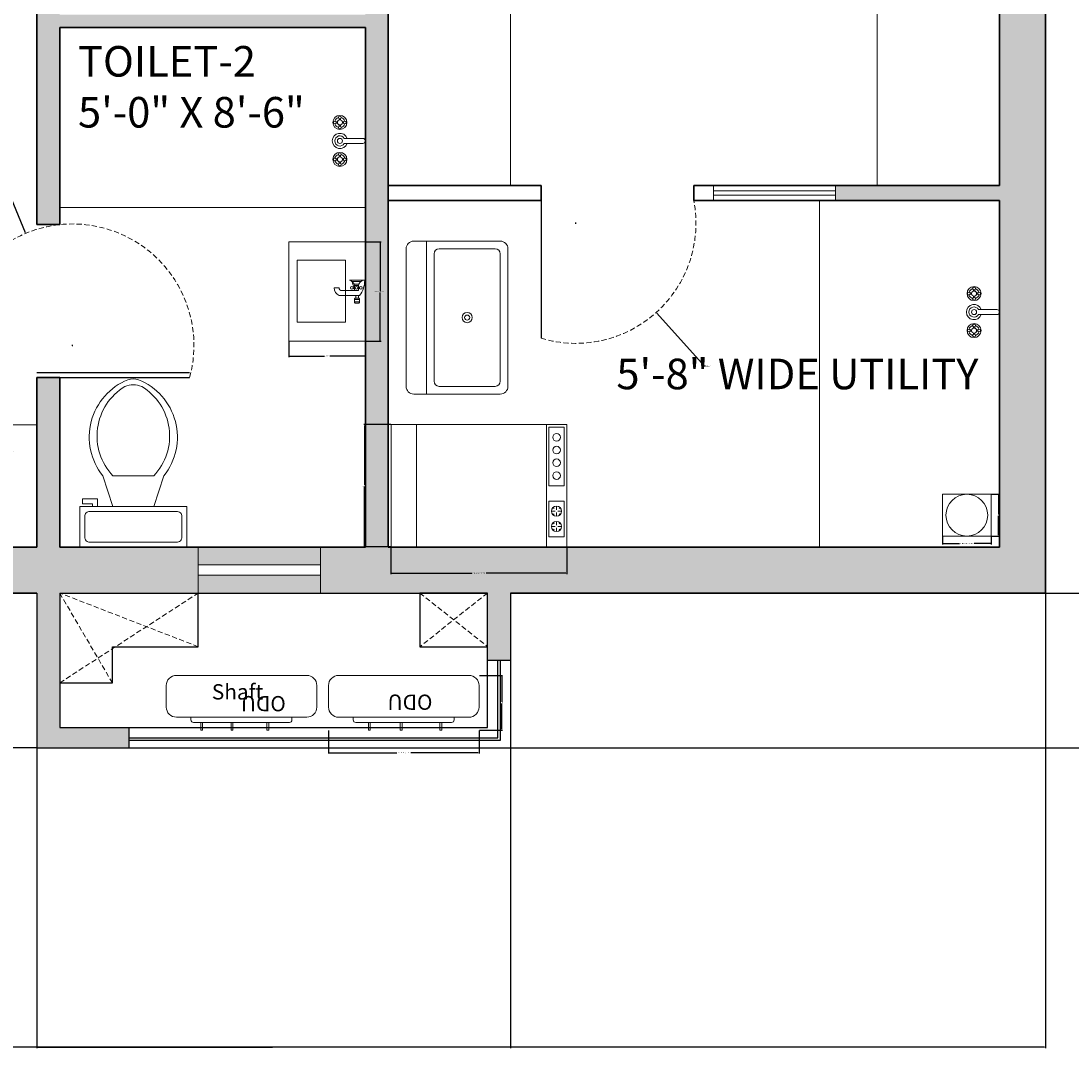
# Model space of a CAD drawing. Units: inches. Extents: x 1693 to 2974, y 2201 to 2965.
# Tile 9 of 24: x 2093 to 2299, y 2201 to 2402. Entities that reach past the tile are written whole.
import ezdxf

# ---------------------------------------------------------------- set-up
doc = ezdxf.new("R2010")
doc.units = ezdxf.units.IN
doc.header["$LTSCALE"] = 2
doc.header["$MEASUREMENT"] = 0
doc.linetypes.add('HIDDEN', pattern=[0.375, 0.25, -0.125])
for name, color, linetype, lineweight in [('A-ANNO-DIMS', 2, 'Continuous', 18), ('A-ANNO-TEXT', 7, 'Continuous', 13), ('A-AREA-IDEN', 7, 'Continuous', 18), ('A-DOOR', 3, 'Continuous', 25), ('A-DOOR-SWNG', 3, 'HIDDEN', 13), ('A-EQPM', 8, 'Continuous', 18), ('A-FLOR-CASE', 32, 'Continuous', 18), ('A-FLOR-FIXT', 9, 'Continuous', 18), ('A-FLOR-SHFT', 7, 'Continuous', 25), ('A-FLOR-SHFT-HIDN', 8, 'HIDDEN', 13), ('A-GLAZ', 4, 'Continuous', 18), ('A-WALL', 7, 'Continuous', 35), ('M-HVAC-EQPM', 151, 'Continuous', 18)]:
    doc.layers.add(name, color=color, linetype=linetype, lineweight=lineweight)
doc.layers.add('A-GLAZ-PATT', color=141, linetype='Continuous', lineweight=13, true_color=0xadddf7)
doc.layers.add('A-WALL-PATT', color=251, linetype='Continuous', lineweight=13, true_color=0x636466)
doc.styles.get("Standard").update_dxf_attribs({"font": 'arial.ttf'})
doc.dimstyles.get("Standard").update_dxf_attribs({"dimtxt": 0.18, "dimasz": 0.18, "dimexe": 0.18, "dimexo": 0.0625, "dimgap": 0.09, "dimtad": 0, "dimtih": 1, "dimtoh": 1, "dimdec": 1, "dimzin": 0, "dimdsep": 46, "dimlunit": 3, "dimtxsty": 'Standard', "dimcen": 0.09, "dimadec": 0, "dimazin": 0, "dimtfac": 1, "dimtdec": 1, "dimtofl": 0, "dimtmove": 0, "dimatfit": 3, "dimfxl": 1, "dimtolj": 1, "dimtzin": 0, "dimarcsym": 0})

# ---------------------------------------------------------------- blocks, each defined once
blk = doc.blocks.new('Faucet - Bathroom top')
for p, q in [((-4.107, 0.125), (-4.375, 0.125)), ((-3.75, 0.4788), (-3.75, 0.75)), ((-3.5, 0.482), (-3.5, 0.75)), ((-3.1461, 0.125), (-2.875, 0.125)), ((3.143, 0.125), (2.875, 0.125)), ((3.5, 0.4788), (3.5, 0.75)), ((3.75, 0.482), (3.75, 0.75)), ((4.1039, 0.125), (4.375, 0.125)), ((-4.1039, -0.125), (-4.375, -0.125)), ((-3.75, -0.4821), (-3.75, -0.75)), ((-3.5, -0.4789), (-3.5, -0.75)), ((-3.143, -0.125), (-2.875, -0.125)), ((-0.5, -0.8639), (-0.5, -4.5)), ((0.5, -4.5), (0.5, -0.8631)), ((3.1461, -0.125), (2.875, -0.125)), ((3.5, -0.4821), (3.5, -0.75)), ((3.75, -0.4789), (3.75, -0.75)), ((4.107, -0.125), (4.375, -0.125))]:
    blk.add_line(p, q)
for centre, radius in [((-3.625, 0), 1.375), ((-4.625, 0), 0.2795), ((-3.625, 0), 0.5), ((-3.625, 1), 0.2795), ((-2.625, 0), 0.2795), ((0, 0), 0.5), ((3.625, 0), 1.375), ((2.625, 0), 0.2795), ((3.625, 0), 0.5), ((3.625, 1), 0.2795), ((4.625, 0), 0.2795), ((-3.625, -1), 0.2795), ((3.625, -1), 0.2795)]:
    blk.add_circle(centre, radius)
for centre, radius, start, end in [((-3.625, 0), 1, 105.2407, 164.2093), ((-3.625, 0), 1, 16.44125, 74.07887), ((0, 0), 1.5, 289.6514, 250.3603), ((0, 0), 1, 300.3431, 239.7554), ((3.625, 0), 1, 106.12, 164.0884), ((3.625, 0), 1, 16.23422, 73.90469), ((-3.625, 0), 1, 196.2342, 253.9047), ((-3.625, 0), 1, 286.12, 344.0884), ((3.625, 0), 1, 196.4413, 254.0789), ((3.625, 0), 1, 285.2407, 344.2093), ((0, -4.5), 0.5, 180, 0)]:
    blk.add_arc(centre, radius, start, end)
blk = doc.blocks.new('Faucet - Bathroom side')
for p, q in [((-0.625, 4.25), (0.375, 4.25)), ((0.375, 3.75), (-0.625, 3.75)), ((-0.625, 3), (3.375, 3)), ((-0.375, 3), (-0.375, 3.5)), ((0.125, 3.5), (0.125, 3)), ((-1.625, 0), (-1.375, 0)), ((-1.375, 0), (1.375, 0)), ((-0.88366, 0.25), (0.88424, 0.25)), ((-0.375, 1.625), (-0.625, 1.625)), ((-0.375, 1.375), (-0.625, 1.375)), ((0.48078, 0.75), (-0.47286, 0.75)), ((2.875, 2), (0.375, 2)), ((0.375, 1.625), (0.625, 1.625)), ((0.375, 1.375), (0.625, 1.375)), ((4.375, 1.5), (3.375, 1.5))]:
    blk.add_line(p, q)
for points in [[(-0.625, 3.75), (-0.625, 4.25)], [(-0.375, 4.5), (0.125, 4.5)], [(0.375, 4.25), (0.375, 3.75)], [(0.125, 3.5), (-0.375, 3.5)]]:
    blk.add_lwpolyline(points)
blk.add_lwpolyline([(-0.375, 1), (-0.375, 2), (0.375, 2), (0.375, 1)], close=True)
for centre in [(-0.875, 1.5), (0, 1.5), (0.875, 1.5)]:
    blk.add_circle(centre, 0.27951)
for centre, radius, start, end in [((-0.38253, 4.2575), 0.24259, 88.22243, 181.7776), ((0.13252, 4.2575), 0.24259, 358.2224, 91.77757), ((3.45929, -0.0281), 5.08436, 143.4467, 179.6834), ((-0.38253, 3.7424), 0.24259, 178.2224, 271.7776), ((0.13252, 3.7424), 0.24259, 268.2224, 1.777565), ((2.70708, 1.4714), 1.66816, 0.9827695, 66.39737), ((-1.75, 1.375), 1.42522, 285.2551, 344.7449), ((1.75, 1.375), 1.42522, 195.2551, 254.7449), ((-2.49562, -0.286), 3.38273, 9.709485, 29.48735), ((2.96867, 1.5936), 0.41699, 347.0192, 102.9808)]:
    blk.add_arc(centre, radius, start, end)
blk = doc.blocks.new('Toilet - top')
for p, q in [((9.5, -6), (9.5, -2)), ((-8, -8.5), (-8, -8)), ((-7, -8), (-7, -9.5)), ((-4, -8), (-6, -14)), ((4, -8), (6, -14)), ((-10, -8.5), (-8, -8.5)), ((-10, -9.5), (-10, -8.5)), ((-7, -9.5), (-10, -9.5)), ((4, -14), (-4, -14))]:
    blk.add_line(p, q)
blk.add_lwpolyline([(10.5, -8), (10.5, 0), (-10.5, 0), (-10.5, -8)], close=True)
for points in [[(-9.5, -2), (-9.5, -6)], [(8.5, -1), (-8.5, -1)], [(-8.5, -7), (8.5, -7)]]:
    blk.add_lwpolyline(points)
for centre, radius, start, end in [((-8.62, -1.88), 0.884, 81.8699, 188.1301), ((8.62, -1.88), 0.884, 351.8699, 98.1301), ((-8.62, -6.12), 0.884, 171.8699, 278.1301), ((8.62, -6.12), 0.884, 261.8699, 8.1301), ((3.52, -21.58), 12.17, 141.4691, 247.9714), ((4.2, -21.82), 11.33, 136.3677, 238.9468), ((-3.52, -21.58), 12.17, 292.0284, 38.5307), ((-4.2, -21.82), 11.33, 301.053, 43.6321), ((0, -27.88), 4, 245.7318, 294.2682), ((0, -29), 4, 254.8605, 285.1395)]:
    blk.add_arc(centre, radius, start, end)
blk = doc.blocks.new('Dishwasher')
for p, q in [((16.3156, 33.1843), (16.5, 33)), ((17, 32.75), (17, 33.5)), ((17.5, 33), (17.6938, 33.1938)), ((19.3156, 33.1843), (19.5, 33)), ((20, 32.75), (20, 33.5)), ((20.5, 33), (20.6938, 33.1938)), ((16, 32.5), (16.75, 32.5)), ((16.5, 32), (16.2942, 31.7942)), ((17, 32.25), (17, 31.5)), ((18, 32.5), (17.25, 32.5)), ((17.7061, 31.7939), (17.5, 32)), ((19, 32.5), (19.75, 32.5)), ((19.5, 32), (19.2942, 31.7942)), ((20, 32.25), (20, 31.5)), ((21, 32.5), (20.25, 32.5)), ((20.7061, 31.7939), (20.5, 32)), ((24, 30.5), (0, 30.5)), ((0, 5), (24, 5))]:
    blk.add_line(p, q)
for points in [[(0, 0), (0, 34.5), (24, 34.5), (24, 0)], [(0.5, 31), (0.5, 34), (12, 34), (12, 31)], [(15, 31), (15, 34), (22, 34), (22, 31)]]:
    blk.add_lwpolyline(points, close=True)
for centre, radius in [((2.5, 32.5), 0.75), ((5, 32.5), 0.75), ((7.5, 32.5), 0.75), ((10, 32.5), 0.75), ((17, 32.5), 1), ((20, 32.5), 1)]:
    blk.add_circle(centre, radius)
blk = doc.blocks.new('Sink-single - 30 in top')
blk.add_line((-15, -3.999996), (15, -3.999996))
for points in [[(-13.5, 0), (13.5, 0)], [(-15, -18.499996), (-15, -1.5)], [(15, -1.5), (15, -18.499996)], [(-12.5, -5.499996), (12.5, -5.499996)], [(-13.5, -17.499996), (-13.5, -6.499996)], [(13.5, -6.499996), (13.5, -17.499996)], [(12.5, -18.499996), (-12.5, -18.499996)], [(13.5, -19.999996), (-13.5, -19.999996)]]:
    blk.add_lwpolyline(points)
for radius in [1, 0.5]:
    blk.add_circle((0, -11.999996), radius)
for centre, radius, start, end in [((-13.5, -1.5), 1.5, 90, 180), ((13.5, -1.5), 1.5, 0, 90), ((-12.5, -6.499996), 1, 90, 180), ((12.5, -6.499996), 1, 0, 90), ((-13.5, -18.499996), 1.5, 180, 270), ((-12.5, -17.499996), 1, 180, 270), ((12.5, -17.499996), 1, 270, 0), ((13.5, -18.499996), 1.5, 270, 0)]:
    blk.add_arc(centre, radius, start, end)
blk = doc.blocks.new('BASIN-WALL-MOUNT')
at = {"ltscale": 2}
for points in [[(15.01, 19.49), (0, 19.49), (0, 0), (15.01, 0)], [(11.1, 15.94), (1.63, 15.94), (1.63, 3.76), (11.1, 3.76)]]:
    blk.add_lwpolyline(points, close=True, dxfattribs=at)
blk = doc.blocks.new('DRAIN-UTILITY')
at = {"ltscale": 2}
blk.add_lwpolyline([(0, 8.21), (9.59, 8.21), (9.59, 0), (0, 0)], close=True, dxfattribs=at)
blk.add_circle((4.8, 4.1), 4.1, dxfattribs=at)
blk = doc.blocks.new('CONDENSER-WITH-BRACKETS')
at = {"ltscale": 2}
for points in [[(2, 10.74), (27.57, 10.74, -0.414214), (29.57, 8.74), (29.57, 4.53, -0.414214), (27.57, 2.53), (2, 2.53, -0.414214), (0, 4.53), (0, 8.74, -0.414214)], [(4.85, 2.53), (24.67, 2.53), (24.67, 2, -0.414214), (24.17, 1.5), (5.35, 1.5, -0.414214), (4.85, 2)]]:
    blk.add_lwpolyline(points, format="xyb", close=True, dxfattribs=at)
for points in [[(7.84, 1.5), (8.19, 1.5), (8.19, 0), (7.84, 0)], [(14.1, 1.5), (14.45, 1.5), (14.45, 0), (14.1, 0)], [(21.89, 1.5), (22.24, 1.5), (22.24, 0), (21.89, 0)]]:
    blk.add_lwpolyline(points, close=True, dxfattribs=at)
blk = doc.blocks.new('*D43')
at = {"layer": 'A-ANNO-DIMS', "color": 0, "lineweight": -2, "ltscale": 2, "transparency": 16777216}
for p, q in [((2160.8, 2358.73), (2163.84, 2358.73)), ((2163.66, 2358.55), (2163.66, 2349.17)), ((2163.66, 2339.42), (2163.66, 2348.8)), ((2160.8, 2339.24), (2163.84, 2339.24))]:
    blk.add_line(p, q, dxfattribs=at)
at = {"layer": 'A-ANNO-DIMS', "color": 0, "ltscale": 2, "transparency": 16777216}
for points in [[(2163.63, 2358.55), (2163.69, 2358.55), (2163.66, 2358.73)], [(2163.63, 2339.42), (2163.69, 2339.42), (2163.66, 2339.24)]]:
    blk.add_solid(points, dxfattribs=at)
at = {"layer": 'Defpoints', "color": 0, "ltscale": 2, "transparency": 16777216}
for p in [(2160.74, 2358.73), (2163.66, 2358.73), (2160.74, 2339.24)]:
    blk.add_point(p, dxfattribs=at)
at = {"layer": 'A-ANNO-DIMS', "color": 0, "ltscale": 2, "transparency": 16777216, "insert": (2163.66, 2348.98), "char_height": 0.18, "attachment_point": 5}
blk.add_mtext('\\A1;WALL BASIN 19 TYP.', dxfattribs=at)
blk = doc.blocks.new('*D44')
at = {"layer": 'A-ANNO-DIMS', "color": 0, "lineweight": -2, "ltscale": 2, "transparency": 16777216}
for p, q in [((2145.72, 2339.18), (2145.72, 2336.13)), ((2160.74, 2339.18), (2160.74, 2336.13)), ((2145.9, 2336.31), (2152.71, 2336.31)), ((2160.56, 2336.31), (2153.75, 2336.31))]:
    blk.add_line(p, q, dxfattribs=at)
at = {"layer": 'A-ANNO-DIMS', "color": 0, "ltscale": 2, "transparency": 16777216}
for points in [[(2145.9, 2336.34), (2145.9, 2336.28), (2145.72, 2336.31)], [(2160.56, 2336.34), (2160.56, 2336.28), (2160.74, 2336.31)]]:
    blk.add_solid(points, dxfattribs=at)
at = {"layer": 'Defpoints', "color": 0, "ltscale": 2, "transparency": 16777216}
for p in [(2145.72, 2339.24), (2160.74, 2339.24), (2160.74, 2336.31)]:
    blk.add_point(p, dxfattribs=at)
at = {"layer": 'A-ANNO-DIMS', "color": 0, "ltscale": 2, "transparency": 16777216, "insert": (2153.23, 2336.31), "char_height": 0.18, "attachment_point": 5}
blk.add_mtext('\\A1;15 TYP.', dxfattribs=at)
blk = doc.blocks.new('*D57')
at = {"layer": 'A-ANNO-DIMS', "color": 0, "lineweight": -2, "ltscale": 2, "transparency": 16777216}
for p, q in [((2165.77, 2298.84), (2165.77, 2293.55)), ((2200.27, 2298.84), (2200.27, 2293.55)), ((2165.95, 2293.73), (2181.61, 2293.73)), ((2200.09, 2293.73), (2184.44, 2293.73))]:
    blk.add_line(p, q, dxfattribs=at)
at = {"layer": 'A-ANNO-DIMS', "color": 0, "ltscale": 2, "transparency": 16777216}
for points in [[(2165.95, 2293.76), (2165.95, 2293.7), (2165.77, 2293.73)], [(2200.09, 2293.76), (2200.09, 2293.7), (2200.27, 2293.73)]]:
    blk.add_solid(points, dxfattribs=at)
at = {"layer": 'Defpoints', "color": 0, "ltscale": 2, "transparency": 16777216}
for p in [(2165.77, 2298.9), (2200.27, 2298.9), (2200.27, 2293.73)]:
    blk.add_point(p, dxfattribs=at)
at = {"layer": 'A-ANNO-DIMS', "color": 0, "ltscale": 2, "transparency": 16777216, "insert": (2183.02, 2293.73), "char_height": 0.18, "attachment_point": 5}
blk.add_mtext('\\A1;DISHWASHER 35 TYP.', dxfattribs=at)
blk = doc.blocks.new('*D58')
at = {"layer": 'A-ANNO-DIMS', "color": 0, "lineweight": -2, "ltscale": 2, "transparency": 16777216}
for p, q in [((2165.71, 2322.9), (2160.42, 2322.9)), ((2160.6, 2322.72), (2160.6, 2311.08)), ((2160.6, 2299.08), (2160.6, 2310.72)), ((2165.71, 2298.9), (2160.42, 2298.9))]:
    blk.add_line(p, q, dxfattribs=at)
at = {"layer": 'A-ANNO-DIMS', "color": 0, "ltscale": 2, "transparency": 16777216}
for points in [[(2160.57, 2322.72), (2160.63, 2322.72), (2160.6, 2322.9)], [(2160.57, 2299.08), (2160.63, 2299.08), (2160.6, 2298.9)]]:
    blk.add_solid(points, dxfattribs=at)
at = {"layer": 'Defpoints', "color": 0, "ltscale": 2, "transparency": 16777216}
for p in [(2165.77, 2322.9), (2160.6, 2298.9), (2165.77, 2298.9)]:
    blk.add_point(p, dxfattribs=at)
at = {"layer": 'A-ANNO-DIMS', "color": 0, "ltscale": 2, "transparency": 16777216, "insert": (2160.6, 2310.9), "char_height": 0.18, "attachment_point": 5}
blk.add_mtext('\\A1;24 TYP.', dxfattribs=at)
blk = doc.blocks.new('*D77')
at = {"layer": 'A-ANNO-DIMS', "color": 0, "lineweight": -2, "ltscale": 2, "transparency": 16777216}
for p, q in [((2274.03, 2300.96), (2274.03, 2299.4)), ((2283.62, 2300.96), (2283.62, 2299.4)), ((2274.21, 2299.58), (2277.37, 2299.58)), ((2283.44, 2299.58), (2280.28, 2299.58))]:
    blk.add_line(p, q, dxfattribs=at)
at = {"layer": 'A-ANNO-DIMS', "color": 0, "ltscale": 2, "transparency": 16777216}
for points in [[(2274.21, 2299.61), (2274.21, 2299.55), (2274.03, 2299.58)], [(2283.44, 2299.61), (2283.44, 2299.55), (2283.62, 2299.58)]]:
    blk.add_solid(points, dxfattribs=at)
at = {"layer": 'Defpoints', "color": 0, "ltscale": 2, "transparency": 16777216}
for p in [(2274.03, 2301.02), (2283.62, 2301.02), (2283.62, 2299.58)]:
    blk.add_point(p, dxfattribs=at)
at = {"layer": 'A-ANNO-DIMS', "color": 0, "ltscale": 2, "transparency": 16777216, "insert": (2278.82, 2299.58), "char_height": 0.18, "attachment_point": 5}
blk.add_mtext('\\A1;UTILITY DRAIN 10 TYP.', dxfattribs=at)
blk = doc.blocks.new('*D78')
at = {"layer": 'A-ANNO-DIMS', "color": 0, "lineweight": -2, "ltscale": 2, "transparency": 16777216}
for p, q in [((2283.68, 2309.23), (2285.24, 2309.23)), ((2285.06, 2309.05), (2285.06, 2305.31)), ((2285.06, 2301.2), (2285.06, 2304.94)), ((2283.68, 2301.02), (2285.24, 2301.02))]:
    blk.add_line(p, q, dxfattribs=at)
at = {"layer": 'A-ANNO-DIMS', "color": 0, "ltscale": 2, "transparency": 16777216}
for points in [[(2285.03, 2309.05), (2285.09, 2309.05), (2285.06, 2309.23)], [(2285.03, 2301.2), (2285.09, 2301.2), (2285.06, 2301.02)]]:
    blk.add_solid(points, dxfattribs=at)
at = {"layer": 'Defpoints', "color": 0, "ltscale": 2, "transparency": 16777216}
for p in [(2283.62, 2309.23), (2285.06, 2309.23), (2283.62, 2301.02)]:
    blk.add_point(p, dxfattribs=at)
at = {"layer": 'A-ANNO-DIMS', "color": 0, "ltscale": 2, "transparency": 16777216, "insert": (2285.06, 2305.12), "char_height": 0.18, "attachment_point": 5}
blk.add_mtext('\\A1;8 TYP.', dxfattribs=at)
blk = doc.blocks.new('*D79')
at = {"layer": 'A-ANNO-DIMS', "color": 0, "lineweight": -2, "ltscale": 2, "transparency": 16777216}
for p, q in [((2153.5, 2262.88), (2153.5, 2258.33)), ((2183.07, 2262.88), (2183.07, 2258.33)), ((2153.68, 2258.51), (2166.92, 2258.51)), ((2182.89, 2258.51), (2169.65, 2258.51))]:
    blk.add_line(p, q, dxfattribs=at)
at = {"layer": 'A-ANNO-DIMS', "color": 0, "ltscale": 2, "transparency": 16777216}
for points in [[(2153.68, 2258.54), (2153.68, 2258.48), (2153.5, 2258.51)], [(2182.89, 2258.54), (2182.89, 2258.48), (2183.07, 2258.51)]]:
    blk.add_solid(points, dxfattribs=at)
at = {"layer": 'Defpoints', "color": 0, "ltscale": 2, "transparency": 16777216}
for p in [(2153.5, 2262.95), (2183.07, 2262.95), (2183.07, 2258.51)]:
    blk.add_point(p, dxfattribs=at)
at = {"layer": 'A-ANNO-DIMS', "color": 0, "ltscale": 2, "transparency": 16777216, "insert": (2168.28, 2258.51), "char_height": 0.18, "attachment_point": 5}
blk.add_mtext('\\A1;CONDENSER 30 TYP.', dxfattribs=at)
blk = doc.blocks.new('*D80')
at = {"layer": 'A-ANNO-DIMS', "color": 0, "lineweight": -2, "ltscale": 2, "transparency": 16777216}
for p, q in [((2183.13, 2273.69), (2187.68, 2273.69)), ((2187.5, 2273.51), (2187.5, 2268.5)), ((2187.5, 2263.13), (2187.5, 2268.14)), ((2183.13, 2262.95), (2187.68, 2262.95))]:
    blk.add_line(p, q, dxfattribs=at)
at = {"layer": 'A-ANNO-DIMS', "color": 0, "ltscale": 2, "transparency": 16777216}
for points in [[(2187.47, 2273.51), (2187.53, 2273.51), (2187.5, 2273.69)], [(2187.47, 2263.13), (2187.53, 2263.13), (2187.5, 2262.95)]]:
    blk.add_solid(points, dxfattribs=at)
at = {"layer": 'Defpoints', "color": 0, "ltscale": 2, "transparency": 16777216}
for p in [(2183.07, 2273.69), (2187.5, 2273.69), (2183.07, 2262.95)]:
    blk.add_point(p, dxfattribs=at)
at = {"layer": 'A-ANNO-DIMS', "color": 0, "ltscale": 2, "transparency": 16777216, "insert": (2187.5, 2268.32), "char_height": 0.18, "attachment_point": 5}
blk.add_mtext('\\A1;11 TYP.', dxfattribs=at)
blk = doc.blocks.new('*D82')
at = {"layer": 'A-ANNO-DIMS', "color": 0, "lineweight": -2, "ltscale": 2, "transparency": 16777216}
for p, q in [((2615.67, 2906.08), (1693.46, 2906.08)), ((1693.64, 2905.9), (1693.64, 2582.94)), ((1693.64, 2259.62), (1693.64, 2582.58)), ((2096.17, 2259.44), (1693.46, 2259.44))]:
    blk.add_line(p, q, dxfattribs=at)
at = {"layer": 'A-ANNO-DIMS', "color": 0, "ltscale": 2, "transparency": 16777216}
for points in [[(1693.61, 2905.9), (1693.67, 2905.9), (1693.64, 2906.08)], [(1693.61, 2259.62), (1693.67, 2259.62), (1693.64, 2259.44)]]:
    blk.add_solid(points, dxfattribs=at)
at = {"layer": 'Defpoints', "color": 0, "ltscale": 2, "transparency": 16777216}
for p in [(1693.64, 2906.08), (2615.74, 2906.08), (2096.24, 2259.44)]:
    blk.add_point(p, dxfattribs=at)
at = {"layer": 'A-ANNO-DIMS', "color": 0, "ltscale": 2, "transparency": 16777216, "insert": (1693.64, 2582.76), "char_height": 0.18, "attachment_point": 5}
blk.add_mtext('\\A1;646.6', dxfattribs=at)
blk = doc.blocks.new('*D83')
at = {"layer": 'A-ANNO-DIMS', "color": 0, "lineweight": -2, "ltscale": 2, "transparency": 16777216}
for p, q in [((1782.74, 2289.78), (1782.74, 2200.56)), ((2294.24, 2289.78), (2294.24, 2200.56)), ((1782.92, 2200.74), (2038.09, 2200.74)), ((2294.06, 2200.74), (2038.88, 2200.74))]:
    blk.add_line(p, q, dxfattribs=at)
at = {"layer": 'A-ANNO-DIMS', "color": 0, "ltscale": 2, "transparency": 16777216}
for points in [[(1782.92, 2200.77), (1782.92, 2200.71), (1782.74, 2200.74)], [(2294.06, 2200.77), (2294.06, 2200.71), (2294.24, 2200.74)]]:
    blk.add_solid(points, dxfattribs=at)
at = {"layer": 'Defpoints', "color": 0, "ltscale": 2, "transparency": 16777216}
for p in [(1782.74, 2289.84), (2294.24, 2289.84), (2294.24, 2200.74)]:
    blk.add_point(p, dxfattribs=at)
at = {"layer": 'A-ANNO-DIMS', "color": 0, "ltscale": 2, "transparency": 16777216, "insert": (2038.49, 2200.74), "char_height": 0.18, "attachment_point": 5}
blk.add_mtext('\\A1;511.5', dxfattribs=at)
blk = doc.blocks.new('*D89')
at = {"layer": 'A-ANNO-DIMS', "color": 0, "lineweight": -2, "ltscale": 2, "transparency": 16777216}
for p, q in [((2479.3, 2334.75), (2973.12, 2334.75)), ((2972.94, 2334.57), (2972.94, 2312.48)), ((2972.94, 2290.02), (2972.94, 2312.12)), ((2294.3, 2289.84), (2973.12, 2289.84))]:
    blk.add_line(p, q, dxfattribs=at)
at = {"layer": 'A-ANNO-DIMS', "color": 0, "ltscale": 2, "transparency": 16777216}
for points in [[(2972.91, 2334.57), (2972.97, 2334.57), (2972.94, 2334.75)], [(2972.91, 2290.02), (2972.97, 2290.02), (2972.94, 2289.84)]]:
    blk.add_solid(points, dxfattribs=at)
at = {"layer": 'Defpoints', "color": 0, "ltscale": 2, "transparency": 16777216}
for p in [(2479.24, 2334.75), (2972.94, 2334.75), (2294.24, 2289.84)]:
    blk.add_point(p, dxfattribs=at)
at = {"layer": 'A-ANNO-DIMS', "color": 0, "ltscale": 2, "transparency": 16777216, "insert": (2972.94, 2312.3), "char_height": 0.18, "attachment_point": 5}
blk.add_mtext('\\A1;44.91', dxfattribs=at)
blk = doc.blocks.new('*D94')
at = {"layer": 'A-ANNO-DIMS', "color": 0, "lineweight": -2, "ltscale": 2, "transparency": 16777216}
for p, q in [((2096.24, 2259.38), (2096.24, 2200.56)), ((2189.24, 2259.38), (2189.24, 2200.56)), ((2096.42, 2200.74), (2142.52, 2200.74)), ((2189.06, 2200.74), (2142.96, 2200.74))]:
    blk.add_line(p, q, dxfattribs=at)
at = {"layer": 'A-ANNO-DIMS', "color": 0, "ltscale": 2, "transparency": 16777216}
for points in [[(2096.42, 2200.77), (2096.42, 2200.71), (2096.24, 2200.74)], [(2189.06, 2200.77), (2189.06, 2200.71), (2189.24, 2200.74)]]:
    blk.add_solid(points, dxfattribs=at)
at = {"layer": 'Defpoints', "color": 0, "ltscale": 2, "transparency": 16777216}
for p in [(2096.24, 2259.44), (2189.24, 2259.44), (2189.24, 2200.74)]:
    blk.add_point(p, dxfattribs=at)
at = {"layer": 'A-ANNO-DIMS', "color": 0, "ltscale": 2, "transparency": 16777216, "insert": (2142.74, 2200.74), "char_height": 0.18, "attachment_point": 5}
blk.add_mtext('\\A1;93', dxfattribs=at)
blk = doc.blocks.new('*D95')
at = {"layer": 'A-ANNO-DIMS', "color": 0, "lineweight": -2, "ltscale": 2, "transparency": 16777216}
for p, q in [((2189.3, 2289.84), (2973.12, 2289.84)), ((2972.94, 2289.66), (2972.94, 2274.83)), ((2972.94, 2259.62), (2972.94, 2274.46)), ((2189.3, 2259.44), (2973.12, 2259.44))]:
    blk.add_line(p, q, dxfattribs=at)
at = {"layer": 'A-ANNO-DIMS', "color": 0, "ltscale": 2, "transparency": 16777216}
for points in [[(2972.91, 2289.66), (2972.97, 2289.66), (2972.94, 2289.84)], [(2972.91, 2259.62), (2972.97, 2259.62), (2972.94, 2259.44)]]:
    blk.add_solid(points, dxfattribs=at)
at = {"layer": 'Defpoints', "color": 0, "ltscale": 2, "transparency": 16777216}
for p in [(2189.24, 2289.84), (2972.94, 2289.84), (2189.24, 2259.44)]:
    blk.add_point(p, dxfattribs=at)
at = {"layer": 'A-ANNO-DIMS', "color": 0, "ltscale": 2, "transparency": 16777216, "insert": (2972.94, 2274.64), "char_height": 0.18, "attachment_point": 5}
blk.add_mtext('\\A1;30.4', dxfattribs=at)
blk = doc.blocks.new('*D126')
at = {"layer": 'A-ANNO-DIMS', "color": 0, "lineweight": -2, "ltscale": 2, "transparency": 16777216}
for p, q in [((2088.31, 2373.6), (2088.49, 2373.6)), ((2088.49, 2373.6), (2093.95, 2360.58)), ((2103.15, 2338.43), (2103.33, 2338.43)), ((2103.24, 2338.34), (2103.24, 2338.52))]:
    blk.add_line(p, q, dxfattribs=at)
at = {"layer": 'A-ANNO-DIMS', "color": 0, "ltscale": 2, "transparency": 16777216}
blk.add_solid([(2093.98, 2360.59), (2093.93, 2360.57), (2094.02, 2360.41)], dxfattribs=at)
at = {"layer": 'Defpoints', "color": 0, "ltscale": 2, "transparency": 16777216}
for p in [(2094.02, 2360.41), (2103.24, 2338.43)]:
    blk.add_point(p, dxfattribs=at)
at = {"layer": 'A-ANNO-DIMS', "color": 0, "ltscale": 2, "transparency": 16777216, "insert": (2087.83, 2373.6), "char_height": 0.18, "attachment_point": 5}
blk.add_mtext('\\A1;R23.84', dxfattribs=at)
blk = doc.blocks.new('*D128')
at = {"layer": 'A-ANNO-DIMS', "color": 0, "lineweight": -2, "ltscale": 2, "transparency": 16777216}
for p, q in [((2201.96, 2362.44), (2202.14, 2362.44)), ((2202.05, 2362.35), (2202.05, 2362.53)), ((2227.31, 2334.37), (2217.96, 2344.77)), ((2227.49, 2334.37), (2227.31, 2334.37))]:
    blk.add_line(p, q, dxfattribs=at)
at = {"layer": 'A-ANNO-DIMS', "color": 0, "ltscale": 2, "transparency": 16777216}
blk.add_solid([(2217.98, 2344.79), (2217.93, 2344.75), (2217.84, 2344.9)], dxfattribs=at)
at = {"layer": 'Defpoints', "color": 0, "ltscale": 2, "transparency": 16777216}
for p in [(2202.05, 2362.44), (2217.84, 2344.9)]:
    blk.add_point(p, dxfattribs=at)
at = {"layer": 'A-ANNO-DIMS', "color": 0, "ltscale": 2, "transparency": 16777216, "insert": (2228.04, 2334.37), "char_height": 0.18, "attachment_point": 5}
blk.add_mtext('\\A1;R23.604', dxfattribs=at)

msp = doc.modelspace()

# ---------------------------------------------------------------- hatches: boundary and pattern name
at = {"layer": 'A-GLAZ-PATT', "ltscale": 2}
h = msp.add_hatch(color=256, dxfattribs=at)
h.dxf.hatch_style = 1
h.paths.add_polyline_path([(2656.9702, 2338.2547), (2632.9702, 2338.2547), (2632.9702, 2339.2547), (2608.9702, 2339.2547), (2608.9702, 2334.7547), (2656.9702, 2334.7547)])
h.paths.add_polyline_path([(2656.9702, 2343.7547), (2608.9702, 2343.7547), (2608.9702, 2340.2547), (2632.9702, 2340.2547), (2632.9702, 2339.2547), (2656.9702, 2339.2547)])
h.paths.add_polyline_path([(2775.7544, 2338.2547), (2751.7544, 2338.2547), (2751.7544, 2334.7547), (2775.7544, 2334.7547)])
h.paths.add_polyline_path([(2775.7544, 2343.7547), (2751.7544, 2343.7547), (2751.7544, 2340.2547), (2775.7544, 2340.2547)])
h.paths.add_polyline_path([(2897.7363, 2568.7999), (2893.2363, 2568.7999), (2893.2363, 2520.7999), (2896.7363, 2520.7999), (2896.7363, 2544.7999), (2897.7363, 2544.7999)])
h.paths.add_polyline_path([(2902.2363, 2568.7999), (2898.7363, 2568.7999), (2898.7363, 2544.7999), (2897.7363, 2544.7999), (2897.7363, 2520.7999), (2902.2363, 2520.7999)])
h.paths.add_polyline_path([(2902.2363, 2637.7547), (2898.7363, 2637.7547), (2898.7363, 2613.7547), (2902.2363, 2613.7547)])
h.paths.add_polyline_path([(2896.7363, 2637.7547), (2893.2363, 2637.7547), (2893.2363, 2613.7547), (2896.7363, 2613.7547)])
h.paths.add_polyline_path([(2902.2363, 2748.903), (2899.0477, 2748.903), (2899.0477, 2724.903), (2898.0477, 2724.903), (2898.0477, 2700.903), (2902.2363, 2700.903)])
h.paths.add_polyline_path([(2898.0477, 2748.903), (2893.2363, 2748.903), (2893.2363, 2700.903), (2897.0477, 2700.903), (2897.0477, 2724.903), (2898.0477, 2724.903)])
h.paths.add_polyline_path([(2851.2363, 2846.2547), (2803.2363, 2846.2547), (2803.2363, 2842.7547), (2827.2363, 2842.7547), (2827.2363, 2841.7547), (2851.2363, 2841.7547)])
h.paths.add_polyline_path([(2851.2363, 2840.7547), (2827.2363, 2840.7547), (2827.2363, 2841.7547), (2803.2363, 2841.7547), (2803.2363, 2837.2547), (2851.2363, 2837.2547)])
h.paths.add_polyline_path([(2578.2363, 2846.2547), (2530.2363, 2846.2547), (2530.2363, 2842.7547), (2554.2363, 2842.7547), (2554.2363, 2841.7547), (2578.2363, 2841.7547)])
h.paths.add_polyline_path([(2578.2363, 2840.7547), (2554.2363, 2840.7547), (2554.2363, 2841.7547), (2530.2363, 2841.7547), (2530.2363, 2837.2547), (2578.2363, 2837.2547)])
h.paths.add_polyline_path([(2732.7363, 2812.7547), (2705.1363, 2812.7547), (2705.1363, 2811.7547), (2676.3363, 2811.7547), (2676.3363, 2812.7547), (2648.7363, 2812.7547), (2648.7363, 2808.2547), (2732.7363, 2808.2547)])
h.paths.add_polyline_path([(2732.7363, 2817.2547), (2648.7363, 2817.2547), (2648.7363, 2813.7547), (2676.3363, 2813.7547), (2676.3363, 2812.7547), (2705.1363, 2812.7547), (2705.1363, 2813.7547), (2732.7363, 2813.7547)])
h.paths.add_polyline_path([(2488.2363, 2695.8203), (2484.7878, 2695.8203), (2484.7878, 2671.8203), (2488.2363, 2671.8203)])
h.paths.add_polyline_path([(2482.7878, 2695.8203), (2479.2363, 2695.8203), (2479.2363, 2671.8203), (2482.7878, 2671.8203)])
h.paths.add_polyline_path([(2488.2363, 2572.4371), (2484.7363, 2572.4371), (2484.7363, 2541.4371), (2483.7363, 2541.4371), (2483.7363, 2512.4371), (2488.2363, 2512.4371)])
h.paths.add_polyline_path([(2482.7363, 2541.4371), (2483.7363, 2541.4371), (2483.7363, 2572.4371), (2479.2363, 2572.4371), (2479.2363, 2512.4371), (2482.7363, 2512.4371)])
h.paths.add_polyline_path([(2248.9863, 2706.8449), (2190.9863, 2706.8449), (2190.9863, 2703.3449), (2219.9863, 2703.3449), (2219.9863, 2702.3449), (2248.9863, 2702.3449)])
h.paths.add_polyline_path([(2248.9863, 2701.3449), (2219.9863, 2701.3449), (2219.9863, 2702.3449), (2190.9863, 2702.3449), (2190.9863, 2697.8449), (2248.9863, 2697.8449)])
h.paths.add_polyline_path([(2151.9207, 2293.3449), (2127.9207, 2293.3449), (2127.9207, 2289.8449), (2151.9207, 2289.8449)])
h.paths.add_polyline_path([(2151.9207, 2298.8449), (2127.9207, 2298.8449), (2127.9207, 2295.3449), (2151.9207, 2295.3449)])
h.paths.add_polyline_path([(2084.023, 2293.3449), (2066.023, 2293.3449), (2066.023, 2294.3449), (2048.023, 2294.3449), (2048.023, 2289.8449), (2084.023, 2289.8449)])
h.paths.add_polyline_path([(2084.023, 2298.8449), (2048.023, 2298.8449), (2048.023, 2295.3449), (2066.023, 2295.3449), (2066.023, 2294.3449), (2084.023, 2294.3449)])
h.paths.add_polyline_path([(1966.0781, 2293.3449), (1948.0781, 2293.3449), (1948.0781, 2294.3449), (1930.0781, 2294.3449), (1930.0781, 2289.8449), (1966.0781, 2289.8449)])
h.paths.add_polyline_path([(1966.0781, 2298.8449), (1930.0781, 2298.8449), (1930.0781, 2295.3449), (1948.0781, 2295.3449), (1948.0781, 2294.3449), (1966.0781, 2294.3449)])
h.paths.add_polyline_path([(1787.2363, 2403.1922), (1782.7363, 2403.1922), (1782.7363, 2355.1922), (1786.2363, 2355.1922), (1786.2363, 2379.1922), (1787.2363, 2379.1922)])
h.paths.add_polyline_path([(1791.7363, 2403.1922), (1788.2363, 2403.1922), (1788.2363, 2379.1922), (1787.2363, 2379.1922), (1787.2363, 2355.1922), (1791.7363, 2355.1922)])
h.paths.add_polyline_path([(1786.2363, 2477.5455), (1782.7363, 2477.5455), (1782.7363, 2453.5455), (1786.2363, 2453.5455)])
h.paths.add_polyline_path([(1791.7363, 2477.5455), (1788.2363, 2477.5455), (1788.2363, 2453.5455), (1791.7363, 2453.5455)])
h.paths.add_polyline_path([(1786.2363, 2621.6433), (1782.7363, 2621.6433), (1782.7363, 2585.6433), (1786.2363, 2585.6433)])
h.paths.add_polyline_path([(1791.7363, 2621.6433), (1788.2363, 2621.6433), (1788.2363, 2585.6433), (1791.7363, 2585.6433)])
h.paths.add_polyline_path([(1908.1286, 2706.8449), (1860.1286, 2706.8449), (1860.1286, 2703.3449), (1884.1286, 2703.3449), (1884.1286, 2702.3449), (1908.1286, 2702.3449)])
h.paths.add_polyline_path([(1908.1286, 2701.3449), (1884.1286, 2701.3449), (1884.1286, 2702.3449), (1860.1286, 2702.3449), (1860.1286, 2697.8449), (1908.1286, 2697.8449)])
h.paths.add_polyline_path([(1973.9863, 2706.8449), (1949.9863, 2706.8449), (1949.9863, 2703.3449), (1973.9863, 2703.3449)])
h.paths.add_polyline_path([(1973.9863, 2701.3449), (1949.9863, 2701.3449), (1949.9863, 2697.8449), (1973.9863, 2697.8449)])
h.paths.add_polyline_path([(2112.7363, 2690.3449), (2028.7363, 2690.3449), (2028.7363, 2686.8449), (2056.3363, 2686.8449), (2056.3363, 2685.8449), (2085.1363, 2685.8449), (2085.1363, 2686.8449), (2112.7363, 2686.8449)])
h.paths.add_polyline_path([(2112.7363, 2685.8449), (2085.1363, 2685.8449), (2085.1363, 2684.8449), (2056.3363, 2684.8449), (2056.3363, 2685.8449), (2028.7363, 2685.8449), (2028.7363, 2681.3449), (2112.7363, 2681.3449)])
h.paths.add_polyline_path([(2422.7363, 2640.7547), (2350.7363, 2640.7547), (2350.7363, 2637.2547), (2386.7363, 2637.2547), (2386.7363, 2636.2547), (2422.7363, 2636.2547)])
h.paths.add_polyline_path([(2422.7363, 2635.2547), (2386.7363, 2635.2547), (2386.7363, 2636.2547), (2350.7363, 2636.2547), (2350.7363, 2631.7547), (2422.7363, 2631.7547)])
at = {"layer": 'A-WALL-PATT', "ltscale": 2}
h = msp.add_hatch(color=256, dxfattribs=at)
h.dxf.hatch_style = 1
h.paths.add_polyline_path([(2294.2363, 2706.8449), (2248.9863, 2706.8449), (2248.9863, 2697.8449), (2285.2363, 2697.8449), (2285.2363, 2586.2648), (2294.2363, 2586.2648)])
h.paths.add_polyline_path([(2294.2363, 2550.2648), (2285.2363, 2550.2648), (2285.2363, 2517.8449), (2141.2363, 2517.8449), (2141.2363, 2513.8449), (2285.2363, 2513.8449), (2285.2363, 2369.8449), (2253.0704, 2369.8449), (2253.0704, 2366.8449), (2285.2363, 2366.8449), (2285.2363, 2298.8449), (2165.2363, 2298.8449), (2165.2363, 2366.8449), (2165.2363, 2369.8449), (2165.2363, 2447.3449), (2160.7363, 2447.3449), (2160.7363, 2403.3449), (2100.7363, 2403.3449), (2100.7363, 2447.3449), (2094.2363, 2447.3449), (2094.2363, 2442.8449), (2096.2363, 2442.8449), (2096.2363, 2362.1344), (2100.7363, 2362.1344), (2100.7363, 2400.8449), (2160.7363, 2400.8449), (2160.7363, 2298.8449), (2151.9207, 2298.8449), (2151.9207, 2289.8449), (2184.7363, 2289.8449), (2184.7363, 2276.6449), (2189.2363, 2276.6449), (2189.2363, 2289.8449), (2294.2363, 2289.8449)])
h.paths.add_polyline_path([(2048.023, 2298.8449), (1976.2363, 2298.8449), (1976.2363, 2442.8449), (2058.2363, 2442.8449, -0.00822734), (2058.2363, 2443.9061), (2058.2363, 2447.3449), (2004.7363, 2447.3449), (1969.7363, 2447.3449), (1969.7363, 2442.8449), (1971.7363, 2442.8449), (1971.7363, 2298.8449), (1966.0781, 2298.8449), (1966.0781, 2289.8449), (2048.023, 2289.8449)])
h.paths.add_polyline_path([(2127.9207, 2298.8449), (2100.7363, 2298.8449), (2100.7363, 2332.1344), (2096.2363, 2332.1344), (2096.2363, 2298.8449), (2084.023, 2298.8449), (2084.023, 2289.8449), (2096.2363, 2289.8449), (2096.2363, 2259.4449), (2114.3201, 2259.4449), (2114.3201, 2263.4449), (2100.7363, 2263.4449), (2100.7363, 2289.8449), (2127.9207, 2289.8449)])

# ---------------------------------------------------------------- linework, layer by layer
at = {"layer": 'A-DOOR', "ltscale": 2}
for p, q in [((2195.2363, 2369.8449), (2195.2363, 2339.8449)), ((2096.2363, 2333.1344), (2126.2363, 2333.1344)), ((2096.2363, 2332.1344), (2126.2363, 2332.1344))]:
    msp.add_line(p, q, dxfattribs=at)
at = {"layer": 'A-DOOR-SWNG', "ltscale": 2}
for centre, radius, start, end in [((2202.0465, 2362.4447), 23.6036, 253.230511, 10.743914), ((2103.2428, 2338.4274), 23.8391, 344.693751, 240.808744)]:
    msp.add_arc(centre, radius, start, end, dxfattribs=at)
at = {"layer": 'A-FLOR-CASE'}
for p, q in [((2261.2363, 2489.8449), (2261.2363, 2369.8449)), ((2189.2363, 2447.3449), (2189.2363, 2369.8449)), ((1976.2363, 2322.8449), (2096.2363, 2322.8449))]:
    msp.add_line(p, q, dxfattribs=at)
at = {"layer": 'A-FLOR-CASE', "ltscale": 2}
for p, q in [((2249.8858, 2366.8449), (2249.8858, 2298.8449)), ((2100.7363, 2365.5049), (2160.7363, 2365.5049))]:
    msp.add_line(p, q, dxfattribs=at)
at = {"layer": 'A-FLOR-SHFT', "ltscale": 2}
for p, q in [((2096.2363, 2289.8449), (2096.2363, 2259.4449)), ((2100.7363, 2289.8449), (2100.7363, 2263.4449)), ((2100.7363, 2289.8449), (2100.7363, 2276.6449)), ((2127.9207, 2279.3136), (2127.9207, 2289.8449)), ((2189.2363, 2289.8449), (2189.2363, 2259.4449)), ((2111.0666, 2272.2041), (2111.0666, 2279.3136)), ((2111.0666, 2279.3136), (2127.9207, 2279.3136)), ((2100.7363, 2276.6449), (2100.7363, 2272.2041)), ((2184.7363, 2276.6449), (2189.2363, 2276.6449)), ((2100.7363, 2272.2041), (2111.0666, 2272.2041)), ((2114.3201, 2263.4449), (2114.3201, 2259.4449)), ((2096.2363, 2259.4449), (2189.2363, 2259.4449))]:
    msp.add_line(p, q, dxfattribs=at)
at = {"layer": 'A-FLOR-SHFT'}
msp.add_line((2100.7363, 2289.8449), (2184.7363, 2289.8449), dxfattribs=at)
at = {"layer": 'A-FLOR-SHFT', "ltscale": 2}
for points in [[(2100.7363, 2263.4449), (2184.7363, 2263.4449), (2184.7363, 2289.8449)], [(2114.3201, 2261.4449), (2186.7363, 2261.4449), (2186.7363, 2276.6449)], [(2114.3201, 2260.9449), (2187.2363, 2260.9449), (2187.2363, 2276.6449)]]:
    msp.add_lwpolyline(points, dxfattribs=at)
msp.add_lwpolyline([(2184.7363, 2289.8449), (2171.4254, 2289.8449), (2171.4254, 2279.3136), (2184.7363, 2279.3136)], close=True, dxfattribs=at)
at = {"layer": 'A-FLOR-SHFT-HIDN', "ltscale": 2}
for p, q in [((2100.7363, 2272.2041), (2127.9207, 2289.8449)), ((2127.9207, 2279.3136), (2100.7363, 2289.8449)), ((2100.7363, 2289.8449), (2111.0666, 2272.2041)), ((2184.7363, 2289.8449), (2171.4254, 2279.3136)), ((2171.4254, 2289.8449), (2184.7363, 2279.3136))]:
    msp.add_line(p, q, dxfattribs=at)
at = {"layer": 'A-GLAZ', "ltscale": 2}
for p, q in [((2229.0704, 2369.8449), (2229.0704, 2366.8449)), ((2253.0704, 2368.7449), (2229.0704, 2368.7449)), ((2253.0704, 2369.8449), (2253.0704, 2366.8449)), ((2253.0704, 2367.9449), (2229.0704, 2367.9449)), ((2127.9207, 2298.8449), (2127.9207, 2289.8449)), ((2151.9207, 2298.8449), (2151.9207, 2289.8449)), ((2127.9207, 2295.3449), (2151.9207, 2295.3449)), ((2127.9207, 2293.3449), (2151.9207, 2293.3449))]:
    msp.add_line(p, q, dxfattribs=at)
at = {"layer": 'A-WALL'}
for p, q in [((2294.2363, 2550.2648), (2294.2363, 2289.8449)), ((2285.2363, 2513.8449), (2285.2363, 2369.8449)), ((2165.2363, 2447.3449), (2165.2363, 2369.8449)), ((2096.2363, 2442.8449), (2096.2363, 2362.1344)), ((2100.7363, 2400.8449), (2160.7363, 2400.8449)), ((2100.7363, 2400.8449), (2100.7363, 2362.1344)), ((2160.7363, 2400.8449), (2160.7363, 2298.8449)), ((2165.2363, 2369.8449), (2195.2363, 2369.8449)), ((2165.2363, 2366.8449), (2165.2363, 2369.8449)), ((2195.2363, 2366.8449), (2195.2363, 2369.8449)), ((2225.2363, 2366.8449), (2225.2363, 2369.8449)), ((2225.2363, 2369.8449), (2285.2363, 2369.8449)), ((2165.2363, 2366.8449), (2195.2363, 2366.8449)), ((2165.2363, 2366.8449), (2165.2363, 2298.8449)), ((2225.2363, 2366.8449), (2285.2363, 2366.8449)), ((2285.2363, 2366.8449), (2285.2363, 2298.8449)), ((2096.2363, 2362.1344), (2100.7363, 2362.1344)), ((2096.2363, 2332.1344), (2100.7363, 2332.1344)), ((2096.2363, 2332.1344), (2096.2363, 2298.8449)), ((2100.7363, 2332.1344), (2100.7363, 2298.8449)), ((1976.2363, 2298.8449), (2096.2363, 2298.8449)), ((2100.7363, 2298.8449), (2160.7363, 2298.8449)), ((2165.2363, 2298.8449), (2285.2363, 2298.8449)), ((1782.7363, 2289.8449), (2096.2363, 2289.8449)), ((2189.2363, 2289.8449), (2294.2363, 2289.8449))]:
    msp.add_line(p, q, dxfattribs=at)
at = {"layer": 'M-HVAC-EQPM', "ltscale": 2}
for points in [[(2123.6436, 2273.6897), (2149.2163, 2273.6897, -0.41421356), (2151.2163, 2271.6897), (2151.2163, 2267.4777, -0.41421356), (2149.2163, 2265.4777), (2123.6436, 2265.4777, -0.41421356), (2121.6436, 2267.4777), (2121.6436, 2271.6897, -0.41421356)], [(2126.4911, 2265.4777), (2146.3127, 2265.4777), (2146.3127, 2264.9426, -0.41421356), (2145.8127, 2264.4426), (2126.9911, 2264.4426, -0.41421356), (2126.4911, 2264.9426)]]:
    msp.add_lwpolyline(points, format="xyb", close=True, dxfattribs=at)
for points in [[(2128.411, 2264.4426), (2128.7644, 2264.4426), (2128.7644, 2262.947), (2128.411, 2262.947)], [(2134.3638, 2264.4426), (2134.7171, 2264.4426), (2134.7171, 2262.947), (2134.3638, 2262.947)], [(2141.4037, 2264.4426), (2141.7571, 2264.4426), (2141.7571, 2262.947), (2141.4037, 2262.947)]]:
    msp.add_lwpolyline(points, close=True, dxfattribs=at)

# ---------------------------------------------------------------- block references
at = {"layer": 'A-EQPM', "ltscale": 2, "rotation": 270}
msp.add_blockref('Dishwasher', (2165.7745, 2322.9023), dxfattribs=at)
at = {"layer": 'A-FLOR-FIXT', "ltscale": 2, "xscale": -1}
for name, p, rotation in [('Faucet - Bathroom top', (2155.7363, 2378.5646), 90), ('Faucet - Bathroom top', (2280.2363, 2344.9774), 90), ('Toilet - top', (2115.1796, 2298.8449), 180)]:
    msp.add_blockref(name, p, dxfattribs=dict(at, rotation=rotation))
at = {"layer": 'A-FLOR-FIXT'}
for name, p in [('BASIN-WALL-MOUNT', (2145.723, 2339.239)), ('DRAIN-UTILITY', (2274.027, 2301.02))]:
    msp.add_blockref(name, p, dxfattribs=at)
at = {"layer": 'A-FLOR-FIXT', "ltscale": 2}
for name, p, rotation in [('Sink-single - 30 in top', (2168.7301, 2343.8978), 90), ('Faucet - Bathroom side', (2158.9863, 2351.2199), 180)]:
    msp.add_blockref(name, p, dxfattribs=dict(at, rotation=rotation))
at = {"layer": 'M-HVAC-EQPM'}
msp.add_blockref('CONDENSER-WITH-BRACKETS', (2153.495, 2262.947), dxfattribs=at)

# ---------------------------------------------------------------- texts
at = {"layer": 'A-ANNO-TEXT', "ltscale": 2, "insert": (2130.5947, 2271.9544), "char_height": 3, "attachment_point": 1}
msp.add_mtext_dynamic_manual_height_columns('Shaft', width=108.452746, gutter_width=1, heights=[0], dxfattribs=at)
at = {"layer": 'A-ANNO-TEXT', "ltscale": 2, "char_height": 3, "attachment_point": 1, "rotation": 180}
for insert in [(2145.1193, 2266.6334), (2173.9094, 2266.9187)]:
    msp.add_mtext_dynamic_manual_height_columns('ODU', width=108.452746, gutter_width=1, heights=[0], dxfattribs=dict(at, insert=insert))
at = {"layer": 'A-AREA-IDEN', "ltscale": 2, "char_height": 6, "attachment_point": 1}
for s, insert in [('TOILET-2\\P5\'-0" X 8\'-6"', (2104.3209, 2397.1878)), ('5\'-8" WIDE UTILITY', (2210.0189, 2335.8332))]:
    msp.add_mtext_dynamic_manual_height_columns(s, width=108.452746, gutter_width=1, heights=[0], dxfattribs=dict(at, insert=insert))

# ---------------------------------------------------------------- dimensions: what is measured, and where the dimension line sits
at = {"layer": 'A-ANNO-DIMS', "ltscale": 2}
for base, p1, p2, override, picture, middle in [((1693.6363, 2906.0761), (2096.2363, 2259.4449), (2615.7363, 2906.0761), {"dimdec": 1, "dimlfac": 1, "dimrnd": 0, "dimzin": 0, "dimdsep": 46, "dimlunit": 2}, '*D82', (1693.6363, 2582.7605)), ((2972.9363, 2334.7547), (2294.2363, 2289.8449), (2479.2363, 2334.7547), {"dimdec": 2, "dimlfac": 1, "dimrnd": 0, "dimzin": 0, "dimdsep": 46, "dimlunit": 2}, '*D89', (2972.9363, 2312.2998)), ((2972.9363, 2289.8449), (2189.2363, 2259.4449), (2189.2363, 2289.8449), {"dimdec": 1, "dimlfac": 1, "dimrnd": 0, "dimzin": 0, "dimdsep": 46, "dimlunit": 2}, '*D95', (2972.9363, 2274.6449))]:
    dim = msp.add_linear_dim(base=base, p1=p1, p2=p2, angle=90, dimstyle='Standard', override=override, dxfattribs=at)
    dim.commit()
    dim.dimension.update_dxf_attribs({"geometry": picture, "text_midpoint": middle})
for center, mpoint, override, picture, middle in [((2103.2428, 2338.4274), (2094.0232, 2360.4116), {"dimdec": 2, "dimlfac": 1, "dimrnd": 0, "dimzin": 0, "dimdsep": 46, "dimlunit": 2}, '*D126', (2087.8319, 2373.6021)), ((2202.0465, 2362.4447), (2217.8361, 2344.8999), {"dimdec": 3, "dimlfac": 1, "dimrnd": 0, "dimzin": 0, "dimdsep": 46, "dimlunit": 2}, '*D128', (2228.0392, 2334.3731))]:
    dim = msp.add_radius_dim(center=center, mpoint=mpoint, dimstyle='Standard', override=override, dxfattribs=at)
    dim.commit()
    dim.dimension.update_dxf_attribs({"geometry": picture, "text_midpoint": middle, "dimtype": 164})
for base, p1, p2, angle, text, picture, middle in [((2163.66, 2358.7303), (2160.7363, 2339.2387), (2160.7363, 2358.7303), 90, 'WALL BASIN <> TYP.', '*D43', (2163.66, 2348.9845)), ((2160.5995, 2298.9023), (2165.7745, 2322.9023), (2165.7745, 2298.9023), 270, '<> TYP.', '*D58', (2160.5995, 2310.9023)), ((2285.0586, 2309.2288), (2283.6197, 2301.0203), (2283.6197, 2309.2288), 90, '<> TYP.', '*D78', (2285.0586, 2305.1245)), ((2187.5042, 2273.6897), (2183.0683, 2262.947), (2183.0683, 2273.6897), 90, '<> TYP.', '*D80', (2187.5042, 2268.3183))]:
    dim = msp.add_linear_dim(base=base, p1=p1, p2=p2, angle=angle, text=text, dimstyle='Standard', override={"dimdec": 0, "dimlfac": 1, "dimrnd": 0, "dimzin": 0, "dimdsep": 46, "dimlunit": 2}, dxfattribs=at)
    dim.commit()
    dim.dimension.update_dxf_attribs({"geometry": picture, "text_midpoint": middle})
for base, p1, p2, text, picture, middle in [((2160.7363, 2336.3149), (2145.7225, 2339.2387), (2160.7363, 2339.2387), '<> TYP.', '*D44', (2153.2294, 2336.3149)), ((2283.6197, 2299.5814), (2274.0269, 2301.0203), (2283.6197, 2301.0203), 'UTILITY DRAIN <> TYP.', '*D77', (2278.8233, 2299.5814)), ((2200.2745145531, 2293.7273190371), (2165.7745145531, 2298.9023190371), (2200.2745145531, 2298.9023190371), 'DISHWASHER <> TYP.', '*D57', (2183.0245145531, 2293.7273190371)), ((2183.0683, 2258.5111), (2153.4955, 2262.947), (2183.0683, 2262.947), 'CONDENSER <> TYP.', '*D79', (2168.2819, 2258.5111))]:
    dim = msp.add_linear_dim(base=base, p1=p1, p2=p2, text=text, dimstyle='Standard', override={"dimdec": 0, "dimlfac": 1, "dimrnd": 0, "dimzin": 0, "dimdsep": 46, "dimlunit": 2}, dxfattribs=at)
    dim.commit()
    dim.dimension.update_dxf_attribs({"geometry": picture, "text_midpoint": middle})
for base, p1, p2, override, picture, middle in [((2294.2363, 2200.7449), (1782.7363, 2289.8449), (2294.2363, 2289.8449), {"dimdec": 1, "dimlfac": 1, "dimrnd": 0, "dimzin": 0, "dimdsep": 46, "dimlunit": 2}, '*D83', (2038.4863, 2200.7449)), ((2189.2363, 2200.7449), (2096.2363, 2259.4449), (2189.2363, 2259.4449), {"dimdec": 0, "dimlfac": 1, "dimrnd": 0, "dimzin": 0, "dimdsep": 46, "dimlunit": 2}, '*D94', (2142.7363, 2200.7449))]:
    dim = msp.add_linear_dim(base=base, p1=p1, p2=p2, dimstyle='Standard', override=override, dxfattribs=at)
    dim.commit()
    dim.dimension.update_dxf_attribs({"geometry": picture, "text_midpoint": middle})

doc.saveas('drawing.dxf')
